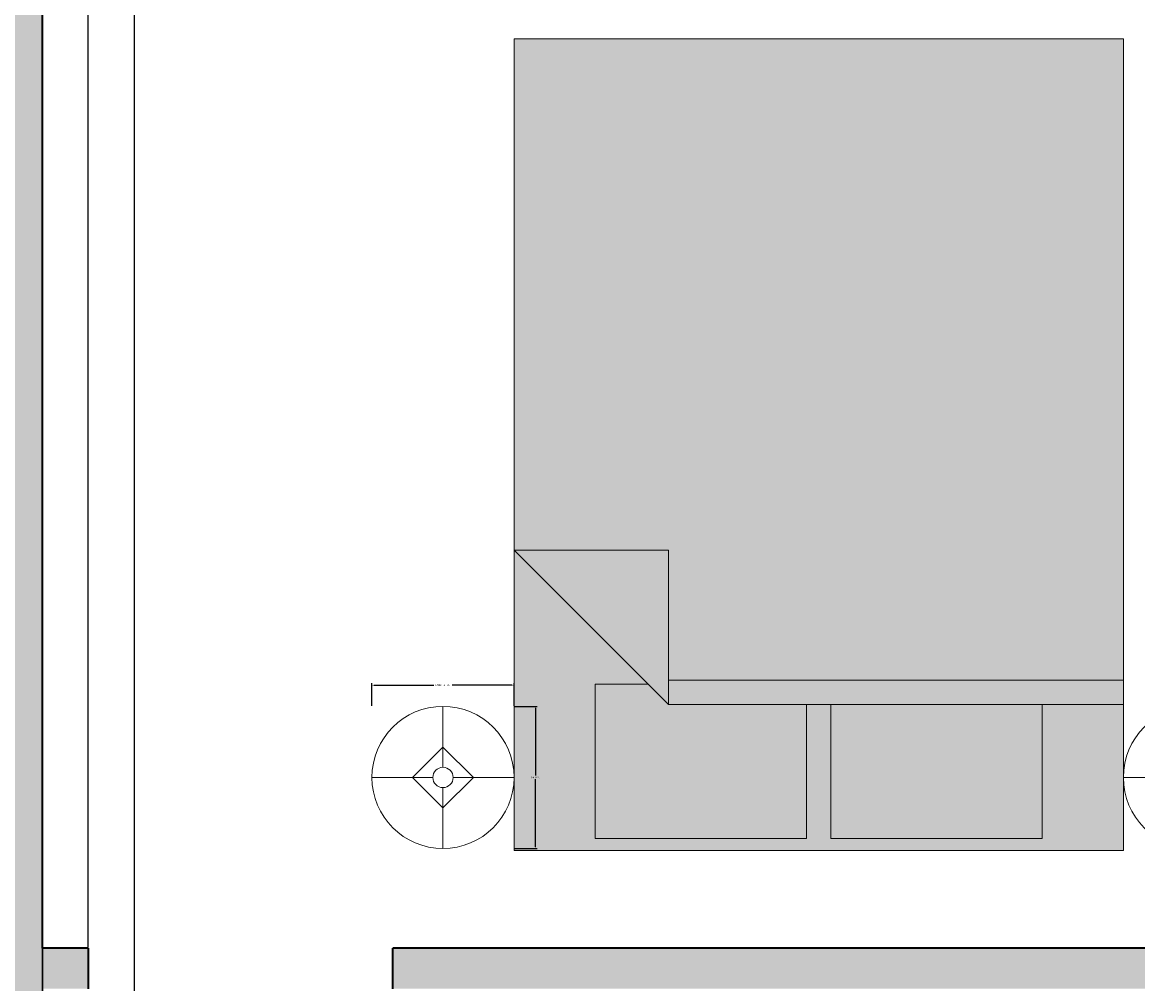
# Model space of a CAD drawing. Units: inches. Extents: x 1567 to 1964, y 1813 to 2447.
# Tile 4 of 28: x 1797 to 1907, y 1964 to 2059. Entities that reach past the tile are written whole.
import ezdxf

# ---------------------------------------------------------------- set-up
doc = ezdxf.new("R2010")
doc.units = ezdxf.units.IN
for name, color, linetype, lineweight in [('A-ANNO-DIMS', 2, 'Continuous', 18), ('A-FURN', 8, 'Continuous', 18), ('A-WALL', 7, 'Continuous', 35)]:
    doc.layers.add(name, color=color, linetype=linetype, lineweight=lineweight)
doc.layers.add('A-FURN-PATT', color=252, linetype='Continuous', lineweight=13, true_color=0x939598)
doc.layers.add('A-WALL-PATT', color=251, linetype='Continuous', lineweight=13, true_color=0x636466)
doc.styles.get("Standard").update_dxf_attribs({"font": 'arial.ttf'})
doc.dimstyles.get("Standard").update_dxf_attribs({"dimtxt": 0.18, "dimasz": 0.18, "dimexe": 0.18, "dimexo": 0.0625, "dimgap": 0.09, "dimtad": 0, "dimtih": 1, "dimtoh": 1, "dimdec": 4, "dimzin": 0, "dimdsep": 46, "dimtxsty": 'Standard', "dimcen": 0.09, "dimadec": 0, "dimazin": 0, "dimtfac": 1, "dimtdec": 4, "dimtofl": 0, "dimtmove": 0, "dimatfit": 3, "dimfxl": 1, "dimtolj": 1, "dimtzin": 0, "dimarcsym": 0})

# ---------------------------------------------------------------- blocks, each defined once
blk = doc.blocks.new('Lamp - Table')
for p, q in [((0, 7), (0, 1)), ((0, 3), (-3, 0)), ((3, 0), (0, 3)), ((-1, 0), (-7, 0)), ((-3, 0), (0, -3)), ((0, -3), (3, 0)), ((1, 0), (7, 0)), ((0, -1), (0, -7))]:
    blk.add_line(p, q)
for radius in [7, 1]:
    blk.add_circle((0, 0), radius)
blk = doc.blocks.new('Bed - Queen')
for p, q in [((0, -80.00003), (0, 0)), ((0, 0), (59.99999, 0)), ((59.99999, 0), (59.99999, -80.00003)), ((7.99999, -1.2), (28.79998, -1.2)), ((7.99999, -14.4), (7.99999, -1.2)), ((28.79998, -1.2), (28.79998, -14.4)), ((31.19999, -1.2), (51.99999, -1.2)), ((31.19999, -14.4), (31.19999, -1.2)), ((51.99999, -1.2), (51.99999, -16.4)), ((0, -14.4), (44.8, -14.4)), ((59.99999, -29.6), (44.8, -14.4)), ((44.8, -14.4), (44.8, -29.6)), ((51.99999, -16.4), (46.79936, -16.4)), ((44.8, -16.8), (0, -16.8)), ((44.8, -29.6), (59.99999, -29.6)), ((59.99999, -80.00003), (0, -80.00003))]:
    blk.add_line(p, q)
blk = doc.blocks.new('*D17')
at = {"layer": 'A-ANNO-DIMS', "color": 0, "lineweight": -2, "transparency": 16777216}
for p, q in [((1831.85, 1991.18), (1831.85, 1993.39)), ((1832.03, 1993.21), (1837.95, 1993.21)), ((1845.67, 1993.21), (1839.75, 1993.21)), ((1845.85, 1991.18), (1845.85, 1993.39))]:
    blk.add_line(p, q, dxfattribs=at)
at = {"layer": 'A-ANNO-DIMS', "color": 0, "transparency": 16777216}
for points in [[(1832.03, 1993.24), (1832.03, 1993.18), (1831.85, 1993.21)], [(1845.67, 1993.24), (1845.67, 1993.18), (1845.85, 1993.21)]]:
    blk.add_solid(points, dxfattribs=at)
at = {"layer": 'Defpoints', "color": 0, "transparency": 16777216}
for p in [(1845.85, 1993.21), (1831.85, 1991.11), (1845.85, 1991.11)]:
    blk.add_point(p, dxfattribs=at)
at = {"layer": 'A-ANNO-DIMS', "color": 0, "transparency": 16777216, "insert": (1838.85, 1993.21), "char_height": 0.18, "attachment_point": 5}
blk.add_mtext('\\A1;LAMP 14 TYP.', dxfattribs=at)
blk = doc.blocks.new('*D18')
at = {"layer": 'A-ANNO-DIMS', "color": 0, "lineweight": -2, "transparency": 16777216}
for p, q in [((1845.92, 1991.11), (1848.13, 1991.11)), ((1847.95, 1990.93), (1847.95, 1984.29)), ((1847.95, 1977.29), (1847.95, 1983.93)), ((1845.92, 1977.11), (1848.13, 1977.11))]:
    blk.add_line(p, q, dxfattribs=at)
at = {"layer": 'A-ANNO-DIMS', "color": 0, "transparency": 16777216}
for points in [[(1847.92, 1990.93), (1847.98, 1990.93), (1847.95, 1991.11)], [(1847.92, 1977.29), (1847.98, 1977.29), (1847.95, 1977.11)]]:
    blk.add_solid(points, dxfattribs=at)
at = {"layer": 'Defpoints', "color": 0, "transparency": 16777216}
for p in [(1845.85, 1991.11), (1845.85, 1977.11), (1847.95, 1977.11)]:
    blk.add_point(p, dxfattribs=at)
at = {"layer": 'A-ANNO-DIMS', "color": 0, "transparency": 16777216, "insert": (1847.95, 1984.11), "char_height": 0.18, "attachment_point": 5}
blk.add_mtext('\\A1;14 TYP.', dxfattribs=at)
blk = doc.blocks.new('*D55')
at = {"layer": 'A-ANNO-DIMS', "color": 0, "lineweight": -2, "transparency": 16777216}
for p, q in [((1795.43, 1964.35), (1795.43, 2447.12)), ((1799.43, 1967.35), (1799.43, 2447.12)), ((1795.61, 2446.94), (1797.28, 2446.94)), ((1799.25, 2446.94), (1797.58, 2446.94))]:
    blk.add_line(p, q, dxfattribs=at)
at = {"layer": 'A-ANNO-DIMS', "color": 0, "transparency": 16777216}
for points in [[(1795.61, 2446.97), (1795.61, 2446.91), (1795.43, 2446.94)], [(1799.25, 2446.97), (1799.25, 2446.91), (1799.43, 2446.94)]]:
    blk.add_solid(points, dxfattribs=at)
at = {"layer": 'Defpoints', "color": 0, "transparency": 16777216}
for p in [(1799.43, 2446.94), (1799.43, 1967.29), (1795.43, 1964.29)]:
    blk.add_point(p, dxfattribs=at)
at = {"layer": 'A-ANNO-DIMS', "color": 0, "transparency": 16777216, "insert": (1797.43, 2446.94), "char_height": 0.18, "attachment_point": 5}
blk.add_mtext('\\A1;4', dxfattribs=at)
blk = doc.blocks.new('*D69')
at = {"layer": 'A-ANNO-DIMS', "color": 0, "lineweight": -2, "transparency": 16777216}
for p, q in [((1799.43, 2123.23), (1799.43, 1813.46)), ((1808.43, 2123.23), (1808.43, 1813.46)), ((1799.61, 1813.64), (1803.78, 1813.64)), ((1808.25, 1813.64), (1804.08, 1813.64))]:
    blk.add_line(p, q, dxfattribs=at)
at = {"layer": 'A-ANNO-DIMS', "color": 0, "transparency": 16777216}
for points in [[(1799.61, 1813.67), (1799.61, 1813.61), (1799.43, 1813.64)], [(1808.25, 1813.67), (1808.25, 1813.61), (1808.43, 1813.64)]]:
    blk.add_solid(points, dxfattribs=at)
at = {"layer": 'Defpoints', "color": 0, "transparency": 16777216}
for p in [(1799.43, 2123.29), (1808.43, 2123.29), (1808.43, 1813.64)]:
    blk.add_point(p, dxfattribs=at)
at = {"layer": 'A-ANNO-DIMS', "color": 0, "transparency": 16777216, "insert": (1803.93, 1813.64), "char_height": 0.18, "attachment_point": 5}
blk.add_mtext('\\A1;9', dxfattribs=at)
blk = doc.blocks.new('*D70')
at = {"layer": 'A-ANNO-DIMS', "color": 0, "lineweight": -2, "transparency": 16777216}
for p, q in [((1799.43, 1967.35), (1799.43, 2447.12)), ((1803.93, 1967.35), (1803.93, 2447.12)), ((1799.61, 2446.94), (1801.42, 2446.94)), ((1803.75, 2446.94), (1801.94, 2446.94))]:
    blk.add_line(p, q, dxfattribs=at)
at = {"layer": 'A-ANNO-DIMS', "color": 0, "transparency": 16777216}
for points in [[(1799.61, 2446.97), (1799.61, 2446.91), (1799.43, 2446.94)], [(1803.75, 2446.97), (1803.75, 2446.91), (1803.93, 2446.94)]]:
    blk.add_solid(points, dxfattribs=at)
at = {"layer": 'Defpoints', "color": 0, "transparency": 16777216}
for p in [(1803.93, 2446.94), (1799.43, 1967.29), (1803.93, 1967.29)]:
    blk.add_point(p, dxfattribs=at)
at = {"layer": 'A-ANNO-DIMS', "color": 0, "transparency": 16777216, "insert": (1801.68, 2446.94), "char_height": 0.18, "attachment_point": 5}
blk.add_mtext('\\A1;4.5', dxfattribs=at)
blk = doc.blocks.new('*D71')
at = {"layer": 'A-ANNO-DIMS', "color": 0, "lineweight": -2, "transparency": 16777216}
for p, q in [((1799.43, 1910.75), (1799.43, 2447.12)), ((1924.43, 1910.75), (1924.43, 2447.12)), ((1799.61, 2446.94), (1861.65, 2446.94)), ((1924.25, 2446.94), (1862.21, 2446.94))]:
    blk.add_line(p, q, dxfattribs=at)
at = {"layer": 'A-ANNO-DIMS', "color": 0, "transparency": 16777216}
for points in [[(1799.61, 2446.97), (1799.61, 2446.91), (1799.43, 2446.94)], [(1924.25, 2446.97), (1924.25, 2446.91), (1924.43, 2446.94)]]:
    blk.add_solid(points, dxfattribs=at)
at = {"layer": 'Defpoints', "color": 0, "transparency": 16777216}
for p in [(1924.43, 2446.94), (1799.43, 1910.69), (1924.43, 1910.69)]:
    blk.add_point(p, dxfattribs=at)
at = {"layer": 'A-ANNO-DIMS', "color": 0, "transparency": 16777216, "insert": (1861.93, 2446.94), "char_height": 0.18, "attachment_point": 5}
blk.add_mtext('\\A1;125', dxfattribs=at)

msp = doc.modelspace()

# ---------------------------------------------------------------- hatches: boundary and pattern name
at = {"layer": 'A-FURN-PATT'}
h = msp.add_hatch(color=256, dxfattribs=at)
h.dxf.hatch_style = 1
h.paths.add_polyline_path([(1621.2532, 2242.0229), (1643.7811, 2241.7239), (1643.8607, 2247.7234), (1617.863, 2248.0685, 0.19047621), (1616.7481, 2164.0759), (1642.7458, 2163.7308), (1642.8254, 2169.7302), (1620.2975, 2170.0293, -0.15194781)])
h.paths.add_polyline_path([(1673.5306, 2249.6607), (1653.8509, 2249.6607), (1653.8509, 2248.5031, 0.11764706), (1673.5306, 2248.5031)])
h.paths.add_polyline_path([(1706.0889, 2249.6607), (1686.4092, 2249.6607), (1686.4092, 2248.5031, 0.11764706), (1706.0889, 2248.5031)])
h.paths.add_polyline_path([(1782.4511, 2227.4197), (1766.4511, 2227.4197), (1766.2949, 2226.4197), (1782.6074, 2226.4197)])
h.paths.add_polyline_path([(1810.4511, 2227.4197), (1794.4511, 2227.4197), (1794.2949, 2226.4197), (1810.6074, 2226.4197)])
h.paths.add_polyline_path([(1743.9511, 2208.076), (1742.9511, 2207.9197), (1742.9511, 2191.9197), (1743.9511, 2191.7635)])
h.paths.add_polyline_path([(1782.6074, 2173.4197), (1766.2949, 2173.4197), (1766.4511, 2172.4197), (1782.4511, 2172.4197)])
h.paths.add_polyline_path([(1810.6074, 2173.4197), (1794.2949, 2173.4197), (1794.4511, 2172.4197), (1810.4511, 2172.4197)])
h.paths.add_polyline_path([(1861.053, 2006.5071), (1845.8531, 2006.5071), (1861.053, 1991.3071)])
h.paths.add_polyline_path([(1905.853, 1993.7071), (1861.053, 1993.7071), (1861.053, 1991.3071), (1905.853, 1991.3071)])
h.paths.add_polyline_path([(1919.7245, 2257.29, 0.50000012), (1918.7245, 2258.29), (1901.7245, 2258.29, 0.50000012), (1900.7245, 2257.29), (1900.7245, 2253.29, 0.50000012), (1901.7245, 2252.29), (1918.7245, 2252.29, 0.50000012), (1919.7245, 2253.29)])
h.paths.add_polyline_path([(1875.9094, 2391.0204), (1875.9094, 2375.8204), (1891.1093, 2375.8204)], flags=17)
h.paths.add_polyline_path([(1891.1093, 2405.4204), (1831.1094, 2405.4204), (1831.1094, 2391.0204), (1839.1093, 2391.0204), (1839.1093, 2404.2204), (1859.9093, 2404.2204), (1859.9093, 2391.0204), (1862.3093, 2391.0204), (1862.3093, 2404.2204), (1883.1093, 2404.2204), (1883.1093, 2389.0204), (1877.9094, 2389.0204), (1891.1093, 2375.8204)])
h.paths.add_polyline_path([(1682.1402, 2390.0316), (1682.1402, 2374.8316), (1697.3402, 2374.8316)], flags=17)
h.paths.add_polyline_path([(1697.3402, 2404.4316), (1637.3402, 2404.4316), (1637.3402, 2390.0316), (1645.3402, 2390.0316), (1645.3402, 2403.2316), (1666.1402, 2403.2316), (1666.1402, 2390.0316), (1668.5402, 2390.0316), (1668.5402, 2403.2316), (1689.3402, 2403.2316), (1689.3402, 2388.0316), (1684.1402, 2388.0316), (1697.3402, 2374.8316)])
h = msp.add_hatch(color=256, dxfattribs=at)
h.dxf.hatch_style = 1
h.paths.add_polyline_path([(1642.2233, 2241.7446), (1623.1648, 2241.9976), (1622.8462, 2217.9997), (1641.9047, 2217.7467)])
h.paths.add_polyline_path([(1641.9047, 2217.7467), (1622.8462, 2217.9997), (1622.5277, 2194.0018), (1641.5862, 2193.7488)])
h.paths.add_polyline_path([(1641.5862, 2193.7488), (1622.5277, 2194.0018), (1622.2091, 2170.0039), (1641.2677, 2169.7509)])
h.paths.add_polyline_path([(1671.2154, 2243.8726, -0.23606798), (1673.5306, 2245.0302), (1673.5306, 2246.1879), (1653.8509, 2246.1879), (1653.8509, 2245.0302, -0.23606798), (1656.1662, 2243.8726), (1656.1662, 2233.4539, -0.23606798), (1653.8509, 2232.2963), (1653.8509, 2231.1387, 0.11764706), (1673.5306, 2231.1387), (1673.5306, 2232.2963, -0.23606798), (1671.2154, 2233.4539)])
h.paths.add_polyline_path([(1703.7736, 2243.8726, -0.23606798), (1706.0889, 2245.0302), (1706.0889, 2246.1879), (1686.4092, 2246.1879), (1686.4092, 2245.0302, -0.23606798), (1688.7245, 2243.8726), (1688.7245, 2233.4539, -0.23606798), (1686.4092, 2232.2963), (1686.4092, 2231.1387, 0.11764706), (1706.0889, 2231.1387), (1706.0889, 2232.2963, -0.23606798), (1703.7736, 2233.4539)])
h.paths.add_polyline_path([(1782.6855, 2225.9197), (1766.2168, 2225.9197), (1764.9668, 2217.9197), (1783.9356, 2217.9197)])
h.paths.add_polyline_path([(1810.6855, 2225.9197), (1794.2168, 2225.9197), (1792.9668, 2217.9197), (1811.9356, 2217.9197)])
h.paths.add_polyline_path([(1752.4511, 2209.4041), (1744.4511, 2208.1541), (1744.4511, 2191.6853), (1752.4511, 2190.4354)])
h.paths.add_polyline_path([(1783.9356, 2181.9197), (1764.9668, 2181.9197), (1766.2168, 2173.9197), (1782.6855, 2173.9197)])
h.paths.add_polyline_path([(1811.9356, 2181.9197), (1792.9668, 2181.9197), (1794.2168, 2173.9197), (1810.6855, 2173.9197)])
h.paths.add_polyline_path([(1832.4511, 2208.1541), (1824.4511, 2209.4041), (1824.4511, 2190.4354), (1832.4511, 2191.6853)])
h.paths.add_polyline_path([(1824.4511, 2194.4197), (1823.8775, 2194.266), (1823.2838, 2194.1743), (1822.6735, 2194.1363), (1822.0501, 2194.1437), (1821.4169, 2194.1882), (1820.7773, 2194.2615), (1820.1348, 2194.3554), (1819.4928, 2194.4614), (1818.8527, 2194.5726), (1818.2083, 2194.6873), (1817.5511, 2194.8049), (1816.873, 2194.9249), (1816.1656, 2195.0469), (1815.4205, 2195.1704), (1814.6296, 2195.2948), (1813.7845, 2195.4197), (1812.88, 2195.5442), (1811.9238, 2195.6658), (1810.9265, 2195.7815), (1809.899, 2195.8885), (1808.852, 2195.9837), (1807.7962, 2196.0643), (1806.7423, 2196.1273), (1805.7011, 2196.1697), (1804.6806, 2196.1896), (1803.6777, 2196.188), (1802.6865, 2196.1668), (1801.7011, 2196.1281), (1800.7158, 2196.0737), (1799.7245, 2196.0057), (1798.7216, 2195.9259), (1797.7011, 2195.8364), (1796.6564, 2195.7387), (1795.5781, 2195.6333), (1794.4557, 2195.52), (1793.2792, 2195.3989), (1792.0383, 2195.27), (1790.7226, 2195.1333), (1789.3219, 2194.9887), (1787.8261, 2194.8364), (1786.1882, 2194.6764), (1784.2148, 2194.5096), (1781.6759, 2194.3369), (1778.3417, 2194.1593), (1773.9821, 2193.9778), (1768.3671, 2193.7934), (1761.2668, 2193.6071), (1752.4511, 2193.4197), (1752.4511, 2189.9197), (1762.0489, 2190.1067), (1769.9836, 2190.2908), (1776.4672, 2190.469), (1781.7115, 2190.6385), (1785.9285, 2190.7962), (1789.33, 2190.9393), (1792.128, 2191.0648), (1794.5344, 2191.1697), (1796.7278, 2191.2521), (1798.7532, 2191.313), (1800.6223, 2191.3543), (1802.3469, 2191.3781), (1803.9387, 2191.3862), (1805.4094, 2191.3807), (1806.7708, 2191.3634), (1808.0345, 2191.3364), (1809.2127, 2191.3013), (1810.3196, 2191.2589), (1811.3699, 2191.2097), (1812.3782, 2191.1541), (1813.3592, 2191.0927), (1814.3274, 2191.0259), (1815.2976, 2190.9542), (1816.2845, 2190.8781), (1817.2985, 2190.7986), (1818.3339, 2190.7186), (1819.3811, 2190.6415), (1820.4303, 2190.5708), (1821.4716, 2190.5098), (1822.4954, 2190.4621), (1823.4918, 2190.4309), (1824.3581, 2190.4208), (1824.4511, 2190.4354)])
h.paths.add_polyline_path([(1874.6531, 1991.3071), (1861.053, 1991.3071), (1859.053, 1993.3071), (1853.8531, 1993.3071), (1853.8531, 1978.1071), (1874.6531, 1978.1071)], flags=17)
h.paths.add_polyline_path([(1897.8531, 1991.3071), (1877.0531, 1991.3071), (1877.0531, 1978.1071), (1897.8531, 1978.1071)], flags=17)
h.paths.add_polyline_path([(1853.8531, 1993.3071), (1859.053, 1993.3071), (1845.8531, 2006.5071), (1845.8531, 1976.9071), (1905.853, 1976.9071), (1905.853, 1991.3071), (1897.8531, 1991.3071), (1897.8531, 1978.1071), (1877.0531, 1978.1071), (1877.0531, 1991.3071), (1874.6531, 1991.3071), (1874.6531, 1978.1071), (1853.8531, 1978.1071)])
h.paths.add_polyline_path([(1920.7245, 2259.29), (1899.7245, 2259.29), (1899.7245, 2251.29), (1920.7245, 2251.29)])
h.paths.add_polyline_path([(1918.7245, 2252.29, 0.50000012), (1919.7245, 2253.29), (1919.7245, 2257.29, 0.50000012), (1918.7245, 2258.29), (1901.7245, 2258.29, 0.50000012), (1900.7245, 2257.29), (1900.7245, 2253.29, 0.50000012), (1901.7245, 2252.29)], flags=16)
h.paths.add_polyline_path([(1843.2327, 2065.967), (1919.26, 2065.967), (1919.26, 2095.8187), (1843.2327, 2095.8187)], flags=9)
h = msp.add_hatch(color=256, dxfattribs=at)
h.dxf.hatch_style = 1
h.paths.add_polyline_path([(1905.853, 2056.9071), (1845.8531, 2056.9071), (1845.8531, 2006.5071), (1861.053, 2006.5071), (1861.053, 1993.7071), (1905.853, 1993.7071)])
at = {"layer": 'A-WALL-PATT'}
h = msp.add_hatch(color=256, dxfattribs=at)
h.dxf.hatch_style = 1
h.paths.add_polyline_path([(1606.4295, 2407.29), (1654.4295, 2407.29), (1654.4295, 2416.29), (1597.4295, 2416.29), (1597.4295, 2217.29), (1606.4295, 2217.29), (1606.4295, 2259.29), (1738.4295, 2259.29), (1738.4295, 2247.29), (1742.4295, 2247.29), (1742.4295, 2259.29), (1742.4295, 2272.29), (1738.4295, 2272.29), (1738.4295, 2263.29), (1606.4295, 2263.29)])
h.paths.add_polyline_path([(1753.4295, 2416.29), (1690.4295, 2416.29), (1690.4295, 2407.29), (1738.4295, 2407.29), (1738.4295, 2308.29), (1742.4295, 2308.29), (1742.4295, 2331.29), (1746.9295, 2331.29), (1746.9295, 2335.29), (1742.4295, 2335.29), (1742.4295, 2407.29), (1753.4295, 2407.29)])
h.paths.add_polyline_path([(1840.4295, 2416.29), (1777.4295, 2416.29), (1777.4295, 2407.29), (1788.4295, 2407.29), (1788.4295, 2335.29), (1776.9295, 2335.29), (1776.9295, 2331.29), (1788.4295, 2331.29), (1788.4295, 2308.29), (1792.4295, 2308.29), (1792.4295, 2407.29), (1840.4295, 2407.29)])
h.paths.add_polyline_path([(1933.4295, 2416.29), (1876.4295, 2416.29), (1876.4295, 2407.29), (1924.4295, 2407.29), (1924.4295, 2263.29), (1792.4295, 2263.29), (1792.4295, 2272.29), (1788.4295, 2272.29), (1788.4295, 2259.29), (1872.4295, 2259.29), (1872.4295, 2171.29), (1880.9295, 2171.29), (1880.9295, 2175.29), (1876.4295, 2175.29), (1876.4295, 2259.29), (1924.4295, 2259.29), (1924.4295, 2229.29), (1933.4295, 2229.29)])
h.paths.add_polyline_path([(1933.4295, 2205.29), (1924.4295, 2205.29), (1924.4295, 2175.29), (1910.9295, 2175.29), (1910.9295, 2171.29), (1924.4295, 2171.29), (1924.4295, 2127.29), (1844.4295, 2127.29), (1844.4295, 2123.29), (1924.4295, 2123.29), (1924.4295, 2063.29), (1933.4295, 2063.29)])
h.paths.add_polyline_path([(1799.4295, 2123.29), (1808.4295, 2123.29), (1808.4295, 2127.29), (1781.4295, 2127.29), (1781.4295, 2123.29), (1795.4295, 2123.29), (1795.4295, 1964.29), (1711.4295, 1964.29), (1711.4295, 2123.29), (1751.4295, 2123.29), (1751.4295, 2127.29), (1742.4295, 2127.29), (1742.4295, 2139.29), (1738.4295, 2139.29), (1738.4295, 2127.29), (1678.4295, 2127.29), (1678.4295, 2123.29), (1702.4295, 2123.29), (1702.4295, 1913.29), (1678.4295, 1913.29), (1678.4295, 1904.29), (1711.4295, 1904.29), (1711.4295, 1960.29), (1795.4295, 1960.29), (1795.4295, 1906.69), (1929.4295, 1906.69), (1929.4295, 1848.29), (1601.4295, 1848.29), (1601.4295, 1904.29), (1630.4295, 1904.29), (1630.4295, 1913.29), (1606.4295, 1913.29), (1606.4295, 2123.29), (1630.4295, 2123.29), (1630.4295, 2127.29), (1606.4295, 2127.29), (1606.4295, 2169.29), (1597.4295, 2169.29), (1597.4295, 1844.29), (1933.4295, 1844.29), (1933.4295, 2027.29), (1924.4295, 2027.29), (1924.4295, 1967.29), (1833.9295, 1967.29), (1833.9295, 1963.29), (1924.4295, 1963.29), (1924.4295, 1910.69), (1799.4295, 1910.69), (1799.4295, 1963.29), (1803.9295, 1963.29), (1803.9295, 1967.29), (1799.4295, 1967.29)])

# ---------------------------------------------------------------- linework, layer by layer
at = {"layer": 'A-WALL'}
for p, q in [((1799.4295, 1967.29), (1799.4295, 2123.29)), ((1803.9295, 1967.29), (1799.4295, 1967.29)), ((1803.9295, 1967.29), (1803.9295, 1963.29)), ((1924.4295, 1967.29), (1833.9295, 1967.29)), ((1833.9295, 1963.29), (1833.9295, 1967.29))]:
    msp.add_line(p, q, dxfattribs=at)

# ---------------------------------------------------------------- block references
at = {"layer": 'A-FURN', "rotation": 180}
for name, p in [('Bed - Queen', (1905.853, 1976.9071)), ('Lamp - Table', (1912.853, 1984.113))]:
    msp.add_blockref(name, p, dxfattribs=at)
at = {"layer": 'A-FURN', "xscale": -1, "rotation": 180}
msp.add_blockref('Lamp - Table', (1838.8531, 1984.113), dxfattribs=at)

# ---------------------------------------------------------------- dimensions: what is measured, and where the dimension line sits
at = {"layer": 'A-ANNO-DIMS'}
for base, p1, p2, override, picture, middle in [((1799.4295, 2446.94), (1795.4295, 1964.29), (1799.4295, 1967.29), {"dimdec": 0, "dimlfac": 1, "dimrnd": 0, "dimzin": 0, "dimdsep": 46, "dimlunit": 2}, '*D55', (1797.4295, 2446.94)), ((1803.9295, 2446.94), (1799.4295, 1967.29), (1803.9295, 1967.29), {"dimdec": 1, "dimlfac": 1, "dimrnd": 0, "dimzin": 0, "dimdsep": 46, "dimlunit": 2}, '*D70', (1801.6795, 2446.94)), ((1924.4295, 2446.94), (1799.4295, 1910.69), (1924.4295, 1910.69), {"dimdec": 0, "dimlfac": 1, "dimrnd": 0, "dimzin": 0, "dimdsep": 46, "dimlunit": 2}, '*D71', (1861.9295, 2446.94)), ((1808.4295, 1813.64), (1799.4295, 2123.29), (1808.4295, 2123.29), {"dimdec": 0, "dimlfac": 1, "dimrnd": 0, "dimzin": 0, "dimdsep": 46, "dimlunit": 2}, '*D69', (1803.9295, 1813.64))]:
    dim = msp.add_linear_dim(base=base, p1=p1, p2=p2, dimstyle='Standard', override=override, dxfattribs=at)
    dim.commit()
    dim.dimension.update_dxf_attribs({"geometry": picture, "text_midpoint": middle})
dim = msp.add_linear_dim(base=(1845.8531, 1993.213), p1=(1831.8531, 1991.113), p2=(1845.8531, 1991.113), text='LAMP <> TYP.', dimstyle='Standard', override={"dimdec": 0, "dimlfac": 1, "dimrnd": 0, "dimzin": 0, "dimdsep": 46, "dimlunit": 2}, dxfattribs=at)
dim.commit()
dim.dimension.update_dxf_attribs({"geometry": '*D17', "text_midpoint": (1838.8531, 1993.213)})
dim = msp.add_linear_dim(base=(1847.9531, 1977.113), p1=(1845.8531, 1991.113), p2=(1845.8531, 1977.113), angle=270, text='<> TYP.', dimstyle='Standard', override={"dimdec": 0, "dimlfac": 1, "dimrnd": 0, "dimzin": 0, "dimdsep": 46, "dimlunit": 2}, dxfattribs=at)
dim.commit()
dim.dimension.update_dxf_attribs({"geometry": '*D18', "text_midpoint": (1847.9531, 1984.113)})

doc.saveas('drawing.dxf')
